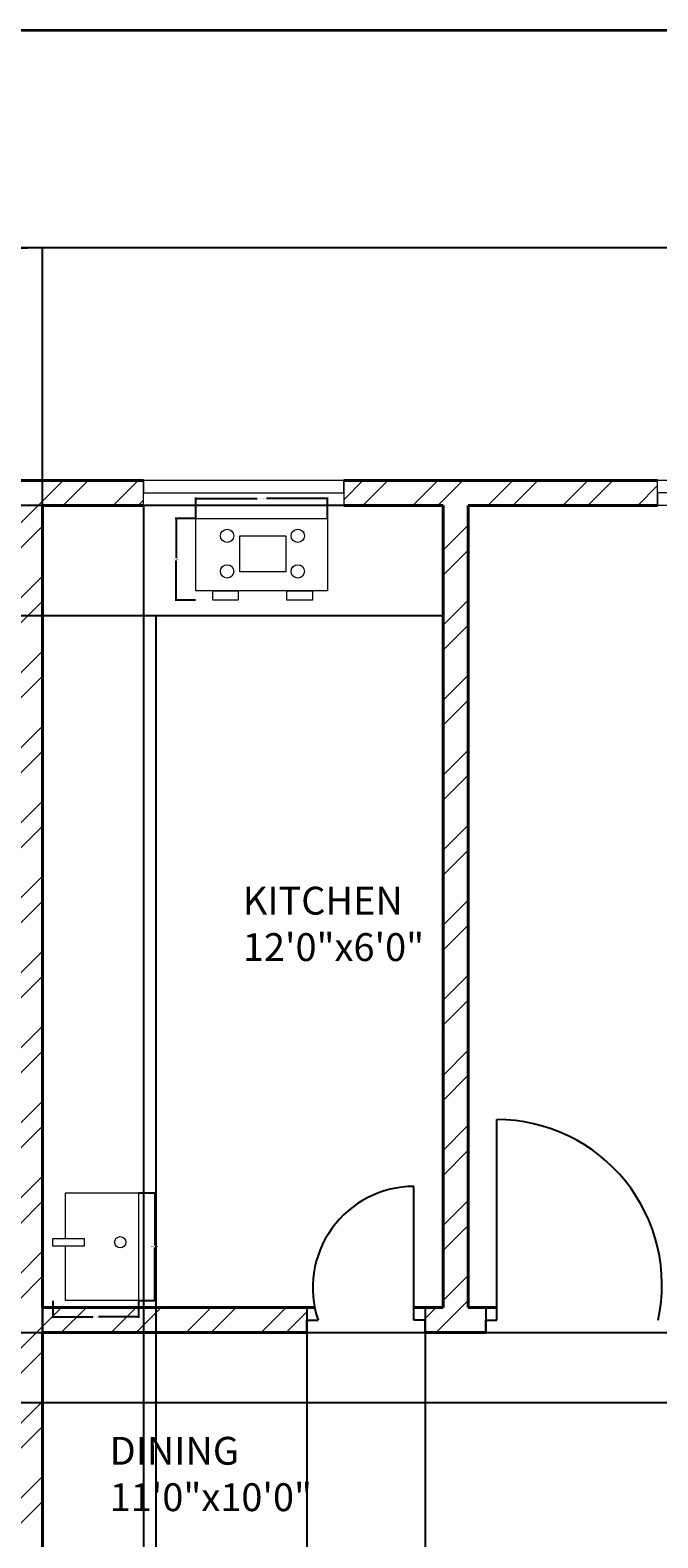
# Model space of a CAD drawing. Units: inches. Extents: x 2063 to 2617, y 1299 to 2210.
# Tile 21 of 22: x 2338 to 2451, y 1939 to 2210. Entities that reach past the tile are written whole.
import ezdxf

# ---------------------------------------------------------------- set-up
doc = ezdxf.new("R2010")
doc.units = ezdxf.units.IN
for name, color, linetype, lineweight in [('A-ANNO-DIMS', 2, 'Continuous', 18), ('A-ANNO-TTLB', 7, 'Continuous', 35), ('A-AREA-IDEN', 7, 'Continuous', 18), ('A-DOOR', 11, 'Continuous', 25), ('A-EQPM', 8, 'Continuous', 18), ('A-FLOR-CASE', 8, 'Continuous', 25), ('A-FLOR-FIXT', 8, 'Continuous', 18), ('A-GLAZ', 123, 'Continuous', 18), ('A-WALL', 7, 'Continuous', 40)]:
    doc.layers.add(name, color=color, linetype=linetype, lineweight=lineweight)
doc.layers.add('A-WALL-PATT', color=215, linetype='Continuous', lineweight=13, true_color=0xa953a0)
doc.styles.get("Standard").update_dxf_attribs({"font": 'arial.ttf'})
doc.dimstyles.get("Standard").update_dxf_attribs({"dimtxt": 0.18, "dimasz": 0.18, "dimexe": 0.18, "dimexo": 0.0625, "dimgap": 0.09, "dimtad": 0, "dimtih": 1, "dimtoh": 1, "dimdec": 4, "dimzin": 0, "dimdsep": 46, "dimtxsty": 'Standard', "dimcen": 0.09, "dimadec": 0, "dimazin": 0, "dimtfac": 1, "dimtdec": 4, "dimtofl": 0, "dimtmove": 0, "dimatfit": 3, "dimfxl": 1, "dimtolj": 1, "dimtzin": 0, "dimarcsym": 0})

# ---------------------------------------------------------------- blocks, each defined once
blk = doc.blocks.new('WIN-60IN')
for p, q in [((0, 60), (4.5, 60)), ((0, 60), (0, 0)), ((4.5, 60), (2.25, 60)), ((2.25, 60), (2.25, 0)), ((4.5, 60), (4.5, 0)), ((2.25, 0), (0, 0)), ((0, 0), (4.5, 0))]:
    blk.add_line(p, q)
blk = doc.blocks.new('WIN-36IN')
for p, q in [((0, 0), (0, 4.5)), ((0, 4.5), (0, 2.25)), ((36, 4.5), (0, 4.5)), ((36, 2.25), (36, 4.5)), ((36, 4.5), (36, 0)), ((0, 2.25), (36, 2.25)), ((0, 0), (36, 0))]:
    blk.add_line(p, q)
blk = doc.blocks.new('COOKTOP-4BURNER')
for points in [[(0, 14.7), (23.64, 14.7), (23.64, 1.68), (0, 1.68)], [(7.88, 11.59), (16.13, 11.59), (16.13, 5.1), (7.88, 5.1)], [(3.01, 1.68), (3.01, 1.68), (3.01, 1.68), (3.01, 1.68)], [(3.01, 1.68), (7.59, 1.68), (7.59, 0), (3.01, 0)], [(16.36, 1.68), (20.94, 1.68), (20.94, 0), (16.36, 0)]]:
    blk.add_lwpolyline(points, close=True)
for centre in [(5.6, 11.57), (18.3, 11.57), (5.6, 5.19), (18.3, 5.19)]:
    blk.add_circle(centre, 1.2)
blk = doc.blocks.new('SINK-SINGLE')
blk.add_lwpolyline([(13.12, 8.22), (13.12, 0), (0, 0), (0, 19.36), (13.12, 19.36), (13.12, 9.57)])
blk.add_lwpolyline([(9.77, 9.57), (15.43, 9.57), (15.43, 8.22), (9.77, 8.22)], close=True)
blk.add_circle((3.31, 8.89), 1.01)
blk = doc.blocks.new('*D21')
at = {"layer": 'A-ANNO-DIMS', "color": 0, "lineweight": -2, "transparency": 16777216}
for p, q in [((2368.2, 2122.06), (2368.2, 2125.72)), ((2368.38, 2125.54), (2379.19, 2125.54)), ((2391.66, 2125.54), (2380.85, 2125.54)), ((2391.84, 2122.06), (2391.84, 2125.72))]:
    blk.add_line(p, q, dxfattribs=at)
at = {"layer": 'A-ANNO-DIMS', "color": 0, "transparency": 16777216}
for points in [[(2368.38, 2125.57), (2368.38, 2125.51), (2368.2, 2125.54)], [(2391.66, 2125.57), (2391.66, 2125.51), (2391.84, 2125.54)]]:
    blk.add_solid(points, dxfattribs=at)
at = {"layer": 'Defpoints', "color": 0, "transparency": 16777216}
for p in [(2391.84, 2125.54), (2368.2, 2121.99), (2391.84, 2121.99)]:
    blk.add_point(p, dxfattribs=at)
at = {"layer": 'A-ANNO-DIMS', "color": 0, "transparency": 16777216, "insert": (2380.02, 2125.54), "char_height": 0.18, "attachment_point": 5}
blk.add_mtext('\\A1;HOB 24 TYP.', dxfattribs=at)
blk = doc.blocks.new('*D22')
at = {"layer": 'A-ANNO-DIMS', "color": 0, "lineweight": -2, "transparency": 16777216}
for p, q in [((2368.14, 2121.99), (2364.48, 2121.99)), ((2364.66, 2121.81), (2364.66, 2114.83)), ((2364.66, 2107.47), (2364.66, 2114.46)), ((2368.14, 2107.29), (2364.48, 2107.29))]:
    blk.add_line(p, q, dxfattribs=at)
at = {"layer": 'A-ANNO-DIMS', "color": 0, "transparency": 16777216}
for points in [[(2364.63, 2121.81), (2364.69, 2121.81), (2364.66, 2121.99)], [(2364.63, 2107.47), (2364.69, 2107.47), (2364.66, 2107.29)]]:
    blk.add_solid(points, dxfattribs=at)
at = {"layer": 'Defpoints', "color": 0, "transparency": 16777216}
for p in [(2364.66, 2121.99), (2368.2, 2121.99), (2368.2, 2107.29)]:
    blk.add_point(p, dxfattribs=at)
at = {"layer": 'A-ANNO-DIMS', "color": 0, "transparency": 16777216, "insert": (2364.66, 2114.64), "char_height": 0.18, "attachment_point": 5}
blk.add_mtext('\\A1;15 TYP.', dxfattribs=at)
blk = doc.blocks.new('*D23')
at = {"layer": 'A-ANNO-DIMS', "color": 0, "lineweight": -2, "transparency": 16777216}
for p, q in [((2357.96, 2000.93), (2360.99, 2000.93)), ((2360.81, 2000.75), (2360.81, 1991.44)), ((2360.81, 1981.75), (2360.81, 1991.07)), ((2357.96, 1981.57), (2360.99, 1981.57))]:
    blk.add_line(p, q, dxfattribs=at)
at = {"layer": 'A-ANNO-DIMS', "color": 0, "transparency": 16777216}
for points in [[(2360.78, 2000.75), (2360.84, 2000.75), (2360.81, 2000.93)], [(2360.78, 1981.75), (2360.84, 1981.75), (2360.81, 1981.57)]]:
    blk.add_solid(points, dxfattribs=at)
at = {"layer": 'Defpoints', "color": 0, "transparency": 16777216}
for p in [(2357.9, 2000.93), (2357.9, 1981.57), (2360.81, 1981.57)]:
    blk.add_point(p, dxfattribs=at)
at = {"layer": 'A-ANNO-DIMS', "color": 0, "transparency": 16777216, "insert": (2360.81, 1991.25), "char_height": 0.18, "attachment_point": 5}
blk.add_mtext('\\A1;SINK 19 TYP.', dxfattribs=at)
blk = doc.blocks.new('*D24')
at = {"layer": 'A-ANNO-DIMS', "color": 0, "lineweight": -2, "transparency": 16777216}
for p, q in [((2342.47, 1981.51), (2342.47, 1978.49)), ((2357.9, 1981.51), (2357.9, 1978.49)), ((2342.65, 1978.67), (2349.67, 1978.67)), ((2357.72, 1978.67), (2350.71, 1978.67))]:
    blk.add_line(p, q, dxfattribs=at)
at = {"layer": 'A-ANNO-DIMS', "color": 0, "transparency": 16777216}
for points in [[(2342.65, 1978.7), (2342.65, 1978.64), (2342.47, 1978.67)], [(2357.72, 1978.7), (2357.72, 1978.64), (2357.9, 1978.67)]]:
    blk.add_solid(points, dxfattribs=at)
at = {"layer": 'Defpoints', "color": 0, "transparency": 16777216}
for p in [(2342.47, 1981.57), (2357.9, 1981.57), (2342.47, 1978.67)]:
    blk.add_point(p, dxfattribs=at)
at = {"layer": 'A-ANNO-DIMS', "color": 0, "transparency": 16777216, "insert": (2350.19, 1978.67), "char_height": 0.18, "attachment_point": 5}
blk.add_mtext('\\A1;15 TYP.', dxfattribs=at)
blk = doc.blocks.new('*D31')
at = {"layer": 'A-ANNO-DIMS', "color": 0, "lineweight": -2, "transparency": 16777216}
for p, q in [((2123.14, 2128.87), (2123.14, 2170.74)), ((2123.32, 2170.56), (2338, 2170.56)), ((2553.46, 2170.56), (2338.79, 2170.56)), ((2553.64, 2128.87), (2553.64, 2170.74))]:
    blk.add_line(p, q, dxfattribs=at)
at = {"layer": 'A-ANNO-DIMS', "color": 0, "transparency": 16777216}
for points in [[(2123.32, 2170.59), (2123.32, 2170.53), (2123.14, 2170.56)], [(2553.46, 2170.59), (2553.46, 2170.53), (2553.64, 2170.56)]]:
    blk.add_solid(points, dxfattribs=at)
at = {"layer": 'Defpoints', "color": 0, "transparency": 16777216}
for p in [(2553.64, 2170.56), (2123.14, 2128.81), (2553.64, 2128.81)]:
    blk.add_point(p, dxfattribs=at)
at = {"layer": 'A-ANNO-DIMS', "color": 0, "transparency": 16777216, "insert": (2338.39, 2170.56), "char_height": 0.18, "attachment_point": 5}
blk.add_mtext('\\A1;430.5', dxfattribs=at)
blk = doc.blocks.new('*D51')
at = {"layer": 'A-ANNO-DIMS', "color": 0, "lineweight": -2, "transparency": 16777216}
for p, q in [((2340.64, 2124.25), (2340.64, 1317.7)), ((2358.75, 2124.25), (2358.75, 1317.7)), ((2340.82, 1317.88), (2349.24, 1317.88)), ((2358.57, 1317.88), (2350.15, 1317.88))]:
    blk.add_line(p, q, dxfattribs=at)
at = {"layer": 'A-ANNO-DIMS', "color": 0, "transparency": 16777216}
for points in [[(2340.82, 1317.91), (2340.82, 1317.85), (2340.64, 1317.88)], [(2358.57, 1317.91), (2358.57, 1317.85), (2358.75, 1317.88)]]:
    blk.add_solid(points, dxfattribs=at)
at = {"layer": 'Defpoints', "color": 0, "transparency": 16777216}
for p in [(2340.64, 2124.31), (2358.75, 2124.31), (2358.75, 1317.88)]:
    blk.add_point(p, dxfattribs=at)
at = {"layer": 'A-ANNO-DIMS', "color": 0, "transparency": 16777216, "insert": (2349.7, 1317.88), "char_height": 0.18, "attachment_point": 5}
blk.add_mtext('\\A1;18.106', dxfattribs=at)
blk = doc.blocks.new('*D53')
at = {"layer": 'A-ANNO-DIMS', "color": 0, "lineweight": -2, "transparency": 16777216}
for p, q in [((2412.58, 2124.31), (2081.21, 2124.31)), ((2081.39, 2124.13), (2081.39, 2114.6)), ((2081.39, 2104.7), (2081.39, 2114.23)), ((2412.58, 2104.52), (2081.21, 2104.52))]:
    blk.add_line(p, q, dxfattribs=at)
at = {"layer": 'A-ANNO-DIMS', "color": 0, "transparency": 16777216}
for points in [[(2081.36, 2124.13), (2081.42, 2124.13), (2081.39, 2124.31)], [(2081.36, 2104.7), (2081.42, 2104.7), (2081.39, 2104.52)]]:
    blk.add_solid(points, dxfattribs=at)
at = {"layer": 'Defpoints', "color": 0, "transparency": 16777216}
for p in [(2412.64, 2124.31), (2081.39, 2104.52), (2412.64, 2104.52)]:
    blk.add_point(p, dxfattribs=at)
at = {"layer": 'A-ANNO-DIMS', "color": 0, "transparency": 16777216, "insert": (2081.39, 2114.42), "char_height": 0.18, "attachment_point": 5}
blk.add_mtext('\\A1;19.792', dxfattribs=at)
blk = doc.blocks.new('*D54')
at = {"layer": 'A-ANNO-DIMS', "color": 0, "lineweight": -2, "transparency": 16777216}
for p, q in [((2340.64, 2124.25), (2340.64, 1317.7)), ((2360.96, 2104.46), (2360.96, 1317.7)), ((2340.82, 1317.88), (2350.34, 1317.88)), ((2360.78, 1317.88), (2351.27, 1317.88))]:
    blk.add_line(p, q, dxfattribs=at)
at = {"layer": 'A-ANNO-DIMS', "color": 0, "transparency": 16777216}
for points in [[(2340.82, 1317.91), (2340.82, 1317.85), (2340.64, 1317.88)], [(2360.78, 1317.91), (2360.78, 1317.85), (2360.96, 1317.88)]]:
    blk.add_solid(points, dxfattribs=at)
at = {"layer": 'Defpoints', "color": 0, "transparency": 16777216}
for p in [(2340.64, 2124.31), (2360.96, 2104.52), (2360.96, 1317.88)]:
    blk.add_point(p, dxfattribs=at)
at = {"layer": 'A-ANNO-DIMS', "color": 0, "transparency": 16777216, "insert": (2350.8, 1317.88), "char_height": 0.18, "attachment_point": 5}
blk.add_mtext('\\A1;20.317', dxfattribs=at)
blk = doc.blocks.new('*D55')
at = {"layer": 'A-ANNO-DIMS', "color": 0, "lineweight": -2, "transparency": 16777216}
for p, q in [((2388.15, 1975.75), (2388.15, 1317.7)), ((2409.37, 1975.75), (2409.37, 1317.7)), ((2388.33, 1317.88), (2398.3, 1317.88)), ((2409.19, 1317.88), (2399.23, 1317.88))]:
    blk.add_line(p, q, dxfattribs=at)
at = {"layer": 'A-ANNO-DIMS', "color": 0, "transparency": 16777216}
for points in [[(2388.33, 1317.91), (2388.33, 1317.85), (2388.15, 1317.88)], [(2409.19, 1317.91), (2409.19, 1317.85), (2409.37, 1317.88)]]:
    blk.add_solid(points, dxfattribs=at)
at = {"layer": 'Defpoints', "color": 0, "transparency": 16777216}
for p in [(2388.15, 1975.81), (2409.37, 1975.81), (2409.37, 1317.88)]:
    blk.add_point(p, dxfattribs=at)
at = {"layer": 'A-ANNO-DIMS', "color": 0, "transparency": 16777216, "insert": (2398.76, 1317.88), "char_height": 0.18, "attachment_point": 5}
blk.add_mtext('\\A1;21.225', dxfattribs=at)
blk = doc.blocks.new('*D59')
at = {"layer": 'A-ANNO-DIMS', "color": 0, "lineweight": -2, "transparency": 16777216}
for p, q in [((2290.14, 1554.56), (2290.14, 2170.74)), ((2290.32, 2170.56), (2315.07, 2170.56)), ((2340.46, 2170.56), (2315.72, 2170.56)), ((2340.64, 1554.56), (2340.64, 2170.74))]:
    blk.add_line(p, q, dxfattribs=at)
at = {"layer": 'A-ANNO-DIMS', "color": 0, "transparency": 16777216}
for points in [[(2290.32, 2170.59), (2290.32, 2170.53), (2290.14, 2170.56)], [(2340.46, 2170.59), (2340.46, 2170.53), (2340.64, 2170.56)]]:
    blk.add_solid(points, dxfattribs=at)
at = {"layer": 'Defpoints', "color": 0, "transparency": 16777216}
for p in [(2340.64, 2170.56), (2290.14, 1554.5), (2340.64, 1554.5)]:
    blk.add_point(p, dxfattribs=at)
at = {"layer": 'A-ANNO-DIMS', "color": 0, "transparency": 16777216, "insert": (2315.39, 2170.56), "char_height": 0.18, "attachment_point": 5}
blk.add_mtext('\\A1;50.5', dxfattribs=at)
blk = doc.blocks.new('*D67')
at = {"layer": 'A-ANNO-DIMS', "color": 0, "lineweight": -2, "transparency": 16777216}
for p, q in [((2127.71, 1975.81), (2595.57, 1975.81)), ((2595.39, 1975.63), (2595.39, 1969.73)), ((2595.39, 1963.46), (2595.39, 1969.36)), ((2128.42, 1963.28), (2595.57, 1963.28))]:
    blk.add_line(p, q, dxfattribs=at)
at = {"layer": 'A-ANNO-DIMS', "color": 0, "transparency": 16777216}
for points in [[(2595.36, 1975.63), (2595.42, 1975.63), (2595.39, 1975.81)], [(2595.36, 1963.46), (2595.42, 1963.46), (2595.39, 1963.28)]]:
    blk.add_solid(points, dxfattribs=at)
at = {"layer": 'Defpoints', "color": 0, "transparency": 16777216}
for p in [(2127.64, 1975.81), (2128.36, 1963.28), (2595.39, 1963.28)]:
    blk.add_point(p, dxfattribs=at)
at = {"layer": 'A-ANNO-DIMS', "color": 0, "transparency": 16777216, "insert": (2595.39, 1969.55), "char_height": 0.18, "attachment_point": 5}
blk.add_mtext('\\A1;12.533', dxfattribs=at)

msp = doc.modelspace()

# ---------------------------------------------------------------- hatches: boundary and pattern name
at = {"layer": 'A-WALL-PATT'}
h = msp.add_hatch(dxfattribs=at)
h.set_pattern_fill('ANSI32', color=256)
h.paths.add_polyline_path([(2127.6442, 2124.3122), (2158.0405, 2124.3122), (2158.0405, 2126.5622), (2158.0405, 2128.8122), (2123.1442, 2128.8122), (2123.1442, 2082.1152), (2127.6442, 2082.1152)])
h.paths.add_polyline_path([(2280.3482, 2128.8122), (2218.0405, 2128.8122), (2218.0405, 2124.3122), (2259.6442, 2124.3122), (2259.6442, 1980.3122), (2256.2494, 1980.3122), (2256.2494, 1975.8122), (2267.1725, 1975.8122), (2267.1725, 1978.0622), (2267.1725, 1980.3122), (2264.1442, 1980.3122), (2264.1442, 2124.3122), (2280.3482, 2124.3122)])
h.paths.add_polyline_path([(2451.1703, 2128.8122), (2394.7501, 2128.8122), (2394.7501, 2124.3122), (2412.6442, 2124.3122), (2412.6442, 1980.3122), (2409.375, 1980.3122), (2409.375, 1975.8122), (2420.2747, 1975.8122), (2420.2747, 1978.0622), (2420.2747, 1980.3122), (2417.1442, 1980.3122), (2417.1442, 2124.3122), (2451.1703, 2124.3122), (2451.1703, 2126.5622)])
h = msp.add_hatch(dxfattribs=at)
h.set_pattern_fill('ANSI32', color=256)
h.paths.add_polyline_path([(2553.6442, 2128.8122), (2511.1703, 2128.8122), (2511.1703, 2124.3122), (2549.1442, 2124.3122), (2549.1442, 2095.662), (2553.6442, 2095.662)])
h.paths.add_polyline_path([(2553.6442, 2035.662), (2549.1442, 2035.662), (2549.1442, 1980.3122), (2503.7214, 1980.3122), (2503.7214, 1975.8122), (2549.1442, 1975.8122), (2549.1442, 1962.9693), (2553.6442, 1962.9693)])
h.paths.add_polyline_path([(2553.6442, 1938.9693), (2549.1442, 1938.9693), (2549.1442, 1927.8122), (2477.1442, 1927.8122), (2477.1442, 1975.8122), (2481.2918, 1975.8122), (2481.2918, 1980.3122), (2453.2648, 1980.3122), (2453.2648, 1975.8122), (2472.6442, 1975.8122), (2472.6442, 1868.3122), (2400.6442, 1868.3122), (2400.6442, 1861.3782), (2405.1442, 1861.3782), (2405.1442, 1863.8122), (2480.9699, 1863.8122), (2480.9699, 1866.0622), (2480.9699, 1868.3122), (2477.1442, 1868.3122), (2477.1442, 1923.3122), (2549.1442, 1923.3122), (2549.1442, 1908.8504), (2553.6442, 1908.8504)])
h.paths.add_polyline_path([(2553.6442, 1884.8504), (2549.1442, 1884.8504), (2549.1442, 1868.3122), (2501.0636, 1868.3122), (2501.0636, 1863.8122), (2549.1442, 1863.8122), (2549.1442, 1826.0298), (2553.6442, 1826.0298)])
h.paths.add_polyline_path([(2388.1504, 1980.3122), (2340.6442, 1980.3122), (2340.6442, 2124.3122), (2358.7501, 2124.3122), (2358.7501, 2128.8122), (2316.3482, 2128.8122), (2316.3482, 2124.3122), (2336.1442, 2124.3122), (2336.1442, 1980.3122), (2289.1737, 1980.3122), (2289.1737, 1975.8122), (2336.1442, 1975.8122), (2336.1442, 1619.3122), (2333.1433, 1619.3122), (2333.1433, 1614.8122), (2344.1671, 1614.8122), (2344.1671, 1617.0622), (2344.1671, 1619.3122), (2340.6442, 1619.3122), (2340.6442, 1975.8122), (2388.1504, 1975.8122), (2388.1504, 1978.0622)])
h.paths.add_polyline_path([(2290.1442, 1614.8122), (2301.4594, 1614.8122), (2301.4594, 1617.0622), (2301.4594, 1619.3122), (2285.6442, 1619.3122), (2285.6442, 1566.8122), (2280.8619, 1566.8122), (2280.8619, 1564.5622), (2280.8619, 1562.3122), (2285.6442, 1562.3122), (2285.6442, 1442.3122), (2281.7879, 1442.3122), (2281.7879, 1437.8122), (2285.6442, 1437.8122), (2285.6442, 1401.8122), (2290.1442, 1401.8122)])
h.paths.add_polyline_path([(2549.1442, 1731.8122), (2405.1442, 1731.8122), (2405.1442, 1834.4638), (2402.8942, 1834.4638), (2400.6442, 1834.4638), (2400.6442, 1727.3122), (2549.1442, 1727.3122)])
h.paths.add_polyline_path([(2553.6442, 1766.0298), (2551.3942, 1766.0298), (2549.1442, 1766.0298), (2549.1442, 1686.7767), (2553.6442, 1686.7767)])
h.paths.add_polyline_path([(2553.6442, 1638.7767), (2551.3942, 1638.7767), (2549.1442, 1638.7767), (2549.1442, 1619.3122), (2448.6442, 1619.3122), (2448.6442, 1610.5671), (2450.8942, 1610.5671), (2453.1442, 1610.5671), (2453.1442, 1614.8122), (2549.1442, 1614.8122), (2549.1442, 1601.6421), (2553.6442, 1601.6421)])
h.paths.add_polyline_path([(2553.6442, 1577.6421), (2551.3942, 1577.6421), (2549.1442, 1577.6421), (2549.1442, 1566.8122), (2453.1442, 1566.8122), (2453.1442, 1591.5045), (2451.0335, 1591.5045), (2448.6442, 1591.5045), (2448.6442, 1566.8122), (2434.0475, 1566.8122), (2434.0475, 1562.3122), (2549.1442, 1562.3122), (2549.1442, 1533.48), (2553.6442, 1533.48)])
h.paths.add_polyline_path([(2553.6442, 1473.48), (2549.1442, 1473.48), (2549.1442, 1442.3122), (2502.6258, 1442.3122), (2502.6258, 1437.8122), (2549.1442, 1437.8122), (2549.1442, 1401.8122), (2553.6442, 1401.8122)])
h.paths.add_polyline_path([(2395.6442, 1562.3122), (2400.0901, 1562.3122), (2400.0901, 1564.5622), (2400.0901, 1566.8122), (2395.6442, 1566.8122), (2395.6442, 1619.3122), (2379.1127, 1619.3122), (2379.1127, 1614.8122), (2391.1442, 1614.8122), (2391.1442, 1401.8122), (2395.6442, 1401.8122), (2395.6442, 1437.8122), (2399.2425, 1437.8122), (2399.2425, 1440.0622), (2399.2425, 1442.3122), (2395.6442, 1442.3122)])
h.paths.add_polyline_path([(2442.6258, 1442.3122), (2419.6262, 1442.3122), (2419.6262, 1437.8122), (2442.6258, 1437.8122), (2442.6258, 1440.0622)])
h.paths.add_polyline_path([(2127.6442, 1480.2532), (2125.3942, 1480.2532), (2123.1442, 1480.2532), (2123.1442, 1401.8122), (2127.6442, 1401.8122), (2127.6442, 1437.8122), (2145.1538, 1437.8122), (2145.1538, 1440.0622), (2145.1538, 1442.3122), (2127.6442, 1442.3122)])
h.paths.add_polyline_path([(2259.809, 1442.3122), (2205.1538, 1442.3122), (2205.1538, 1437.8122), (2259.809, 1437.8122), (2259.809, 1440.0622)])
h.paths.add_polyline_path([(2127.6442, 1659.7652), (2123.1442, 1659.7652), (2123.1442, 1605.5161), (2125.3942, 1605.5161), (2127.6442, 1605.5161), (2127.6442, 1614.8122), (2223.6442, 1614.8122), (2223.6442, 1611.2723), (2228.1442, 1611.2723), (2228.1442, 1619.3122), (2127.6442, 1619.3122)])
h.paths.add_polyline_path([(2244.8673, 1566.8122), (2228.1442, 1566.8122), (2228.1442, 1590.8122), (2225.8942, 1590.8122), (2223.6442, 1590.8122), (2223.6442, 1566.8122), (2127.6442, 1566.8122), (2127.6442, 1581.5161), (2123.1442, 1581.5161), (2123.1442, 1540.2532), (2127.6442, 1540.2532), (2127.6442, 1562.3122), (2244.8673, 1562.3122), (2244.8673, 1564.5622)])
h.paths.add_polyline_path([(2172.5174, 1868.3122), (2127.6442, 1868.3122), (2127.6442, 1886.5833), (2123.1442, 1886.5833), (2123.1442, 1832.6633), (2127.6442, 1832.6633), (2127.6442, 1863.8122), (2172.5174, 1863.8122), (2172.5174, 1866.0622)])
h.paths.add_polyline_path([(2276.1442, 1868.3122), (2204.1442, 1868.3122), (2204.1442, 1923.3122), (2204.1442, 1975.8122), (2224.8362, 1975.8122), (2224.8362, 1978.1097), (2224.8362, 1980.3122), (2195.0729, 1980.3122), (2195.0729, 1978.0622), (2195.0729, 1975.8122), (2199.6442, 1975.8122), (2199.6442, 1927.8122), (2127.6442, 1927.8122), (2127.6442, 1942.3492), (2123.1442, 1942.3492), (2123.1442, 1910.5833), (2127.6442, 1910.5833), (2127.6442, 1923.3122), (2199.6442, 1923.3122), (2199.6442, 1868.3122), (2194.8228, 1868.3122), (2194.8228, 1864.7337), (2194.8228, 1863.8122), (2271.6442, 1863.8122), (2271.6442, 1860.0507), (2276.1442, 1860.0507)])
h.paths.add_polyline_path([(2276.1442, 1829.994), (2273.8942, 1829.994), (2271.6442, 1829.994), (2271.6442, 1731.8122), (2127.6442, 1731.8122), (2127.6442, 1772.6633), (2123.1442, 1772.6633), (2123.1442, 1707.7652), (2127.6442, 1707.7652), (2127.6442, 1727.3122), (2276.1442, 1727.3122)])
h.paths.add_polyline_path([(2127.6442, 2022.1152), (2123.1442, 2022.1152), (2123.1442, 1966.3492), (2127.6442, 1966.3492), (2127.6442, 1975.8122), (2174.2082, 1975.8122), (2174.2082, 1978.0622), (2174.2082, 1980.3122), (2127.6442, 1980.3122)])
h.paths.add_polyline_path([(2361.9755, 1678.588), (2398.4558, 1678.588), (2398.4558, 1697.2453), (2361.9755, 1697.2453)], flags=9)
h.paths.add_polyline_path([(2351.5397, 1780.4072), (2386.1987, 1780.4072), (2386.1987, 1790.7107), (2351.5397, 1790.7107)], flags=25)
h.paths.add_polyline_path([(2350.6753, 1940.9321), (2387.6024, 1940.9321), (2387.6024, 1959.5894), (2350.6753, 1959.5894)], flags=25)
h.paths.add_polyline_path([(2254.9545, 1684.638), (2295.0943, 1684.638), (2295.0943, 1703.2953), (2254.9545, 1703.2953)], flags=9)
h.paths.add_polyline_path([(2282.4946, 1782.4438), (2317.1535, 1782.4438), (2317.1535, 1792.7474), (2282.4946, 1792.7474)], flags=9)
h.paths.add_polyline_path([(2270.327, 1939.2854), (2307.254, 1939.2854), (2307.254, 1957.9428), (2270.327, 1957.9428)], flags=9)

# ---------------------------------------------------------------- linework, layer by layer
at = {"layer": 'A-ANNO-TTLB'}
msp.add_lwpolyline([(2062.5792, 2209.6485), (2617.0648, 2209.6485), (2617.0648, 1299.1125), (2062.5792, 1299.1125)], close=True, dxfattribs=at)
at = {"layer": 'A-DOOR'}
for p, q in [((2422.2747, 1978.0622), (2422.2747, 2014.0622)), ((2407.375, 1978.0622), (2407.375, 2002.0622)), ((2388.1504, 1980.3122), (2388.1504, 1975.8122)), ((2409.375, 1980.3122), (2409.375, 1975.8122)), ((2420.2747, 1980.3122), (2420.2747, 1975.8122)), ((2388.1504, 1975.8122), (2388.1504, 1978.0622)), ((2388.1504, 1978.0622), (2390.1504, 1978.0622)), ((2409.375, 1978.0622), (2407.375, 1978.0622)), ((2409.375, 1975.8122), (2409.375, 1978.0622)), ((2420.2747, 1975.8122), (2420.2747, 1978.0622)), ((2420.2747, 1978.0622), (2422.2747, 1978.0622))]:
    msp.add_line(p, q, dxfattribs=at)
for centre, radius, start, end in [((2422.2747, 1984.3896), 29.6726, 347.687693, 90), ((2407.375, 1983.8813), 18.1809, 90, 198.666862)]:
    msp.add_arc(centre, radius, start, end, dxfattribs=at)
at = {"layer": 'A-FLOR-CASE'}
for p, q in [((2412.6442, 2104.5201), (2360.9612, 2104.5201)), ((2360.9612, 2104.5201), (2360.9612, 1980.3122))]:
    msp.add_line(p, q, dxfattribs=at)
at = {"layer": 'A-WALL'}
for p, q in [((2316.3482, 2128.8122), (2358.7501, 2128.8122)), ((2316.3482, 2128.8122), (2358.7501, 2128.8122)), ((2394.7501, 2128.8122), (2451.1703, 2128.8122)), ((2394.7501, 2128.8122), (2451.1703, 2128.8122)), ((2340.6442, 2124.3122), (2340.6442, 1980.3122)), ((2340.6442, 2124.3122), (2358.7501, 2124.3122)), ((2394.7501, 2124.3122), (2412.6442, 2124.3122)), ((2412.6442, 2124.3122), (2412.6442, 1980.3122)), ((2417.1442, 2124.3122), (2417.1442, 1980.3122)), ((2417.1442, 2124.3122), (2451.1703, 2124.3122)), ((2340.6442, 1980.3122), (2389.5478, 1980.3122)), ((2407.375, 1980.3122), (2412.6442, 1980.3122)), ((2417.1442, 1980.3122), (2422.2747, 1980.3122)), ((2340.6442, 1975.8122), (2340.6442, 1619.3122)), ((2340.6442, 1975.8122), (2388.1504, 1975.8122)), ((2409.375, 1975.8122), (2420.2747, 1975.8122))]:
    msp.add_line(p, q, dxfattribs=at)

# ---------------------------------------------------------------- block references
at = {"layer": 'A-EQPM'}
msp.add_blockref('COOKTOP-4BURNER', (2368.201, 2107.294), dxfattribs=at)
at = {"layer": 'A-FLOR-FIXT', "rotation": 180}
msp.add_blockref('SINK-SINGLE', (2357.9013, 2000.9332), dxfattribs=at)
at = {"layer": 'A-GLAZ'}
msp.add_blockref('WIN-36IN', (2358.7499, 2124.312), dxfattribs=at)
at = {"layer": 'A-GLAZ', "extrusion": (0, 0, -1), "zscale": -1, "rotation": 90}
msp.add_blockref('WIN-60IN', (-2451.1701, 2124.3119), dxfattribs=at)

# ---------------------------------------------------------------- texts
at = {"layer": 'A-AREA-IDEN', "char_height": 5, "attachment_point": 1}
for s, width, insert in [('KITCHEN\\P12\'0"x6\'0"', 190.311974, (2376.6228, 2055.8619)), ('DINING\\P11\'0"x10\'0"', 164.404881, (2352.6859, 1957.1013))]:
    msp.add_mtext_dynamic_manual_height_columns(s, width=width, gutter_width=12.5, heights=[0], dxfattribs=dict(at, insert=insert))

# ---------------------------------------------------------------- dimensions: what is measured, and where the dimension line sits
at = {"layer": 'A-ANNO-DIMS'}
for base, p1, p2, override, picture, middle in [((2553.6442, 2170.5622), (2123.1442, 2128.8122), (2553.6442, 2128.8122), {"dimdec": 1, "dimlfac": 1, "dimrnd": 0, "dimzin": 0, "dimdsep": 46, "dimlunit": 2}, '*D31', (2338.3942, 2170.5622)), ((2340.6442, 2170.5622), (2290.1442, 1554.4994), (2340.6442, 1554.4994), {"dimdec": 1, "dimlfac": 1, "dimrnd": 0, "dimzin": 0, "dimdsep": 46, "dimlunit": 2}, '*D59', (2315.3942, 2170.5622)), ((2358.7501, 1317.8821), (2340.6442, 2124.3122), (2358.7501, 2124.3122), {"dimdec": 3, "dimlfac": 1, "dimrnd": 0, "dimzin": 0, "dimdsep": 46, "dimlunit": 2}, '*D51', (2349.6972, 1317.8821)), ((2360.9612, 1317.8821), (2340.6442, 2124.3122), (2360.9612, 2104.5201), {"dimdec": 3, "dimlfac": 1, "dimrnd": 0, "dimzin": 0, "dimdsep": 46, "dimlunit": 2}, '*D54', (2350.8027, 1317.8821)), ((2409.375, 1317.8821), (2388.1504, 1975.8122), (2409.375, 1975.8122), {"dimdec": 3, "dimlfac": 1, "dimrnd": 0, "dimzin": 0, "dimdsep": 46, "dimlunit": 2}, '*D55', (2398.7627, 1317.8821))]:
    dim = msp.add_linear_dim(base=base, p1=p1, p2=p2, dimstyle='Standard', override=override, dxfattribs=at)
    dim.commit()
    dim.dimension.update_dxf_attribs({"geometry": picture, "text_midpoint": middle})
dim = msp.add_linear_dim(base=(2391.8372, 2125.5381), p1=(2368.2008, 2121.9926), p2=(2391.8372, 2121.9926), text='HOB <> TYP.', dimstyle='Standard', override={"dimdec": 0, "dimlfac": 1, "dimrnd": 0, "dimzin": 0, "dimdsep": 46, "dimlunit": 2}, dxfattribs=at)
dim.commit()
dim.dimension.update_dxf_attribs({"geometry": '*D21', "text_midpoint": (2380.019, 2125.5381)})
for base, p1, p2, picture, middle in [((2081.3943, 2104.5201), (2412.6442, 2124.3122), (2412.6442, 2104.5201), '*D53', (2081.3943, 2114.4162)), ((2595.3943, 1963.2791), (2127.6442, 1975.8122), (2128.3589, 1963.2791), '*D67', (2595.3943, 1969.5457))]:
    dim = msp.add_linear_dim(base=base, p1=p1, p2=p2, angle=90, dimstyle='Standard', override={"dimdec": 3, "dimlfac": 1, "dimrnd": 0, "dimzin": 0, "dimdsep": 46, "dimlunit": 2}, dxfattribs=at)
    dim.commit()
    dim.dimension.update_dxf_attribs({"geometry": picture, "text_midpoint": middle})
for base, p1, p2, angle, text, picture, middle in [((2364.6554, 2121.9926), (2368.2008, 2107.2937), (2368.2008, 2121.9926), 90, '<> TYP.', '*D22', (2364.6554, 2114.6432)), ((2360.8052, 1981.5722), (2357.9011, 2000.9331), (2357.9011, 1981.5722), 270, 'SINK <> TYP.', '*D23', (2360.8052, 1991.2526)), ((2342.4701, 1978.668), (2357.9011, 1981.5722), (2342.4701, 1981.5722), 180, '<> TYP.', '*D24', (2350.1856, 1978.668))]:
    dim = msp.add_linear_dim(base=base, p1=p1, p2=p2, angle=angle, text=text, dimstyle='Standard', override={"dimdec": 0, "dimlfac": 1, "dimrnd": 0, "dimzin": 0, "dimdsep": 46, "dimlunit": 2}, dxfattribs=at)
    dim.commit()
    dim.dimension.update_dxf_attribs({"geometry": picture, "text_midpoint": middle})

doc.saveas('drawing.dxf')
